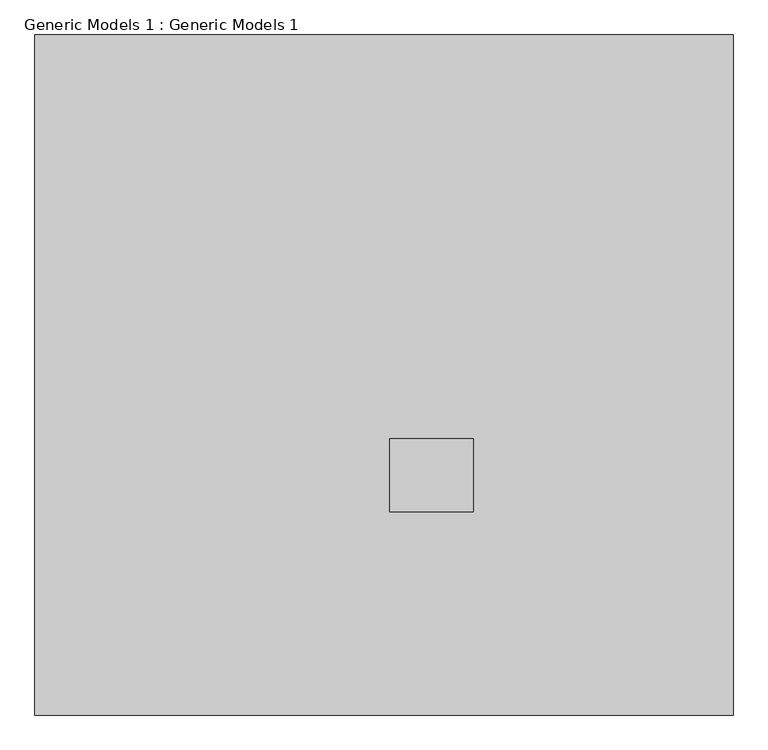
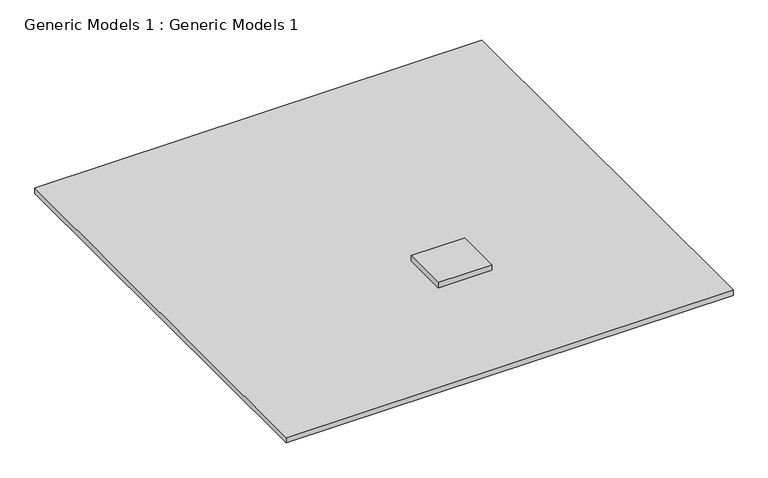
"""IFC4 building model written with IfcOpenShell, lengths in millimetres: proxy geometry, Generic Models 1 : Generic Models 1."""

from ifc_helpers import new_model, si_unit, frame, origin, origin_with_axes, place, context, project, spatial, polyline, outline, extrude, source, transform, mapped, element, save


def generic_models_1_generic_models_1_010c0d49(model_context):
    return source(origin(), model_context, "Body", "SweptSolid", [
        extrude(outline(polyline([(1074.6746771, 1256.1715228), (1074.6746771, -21706.0341115), (-22498.0233478, -21706.0341115), (-22498.0233478, 1256.1715228), (1074.6746771, 1256.1715228)])), frame((0.0, 0.0, -304.8), z_axis=(0.0, 0.0, 1.0), x_axis=(1.0, 0.0, 0.0)), (0.0, 0.0, 1.0), 304.8),
        extrude(outline(polyline([(-7700.6281629, -12372.4678064), (-7700.6281629, -14848.9678064), (-10520.0281629, -14848.9678064), (-10520.0281629, -12372.4678064), (-7700.6281629, -12372.4678064)])), origin_with_axes(), (0.0, 0.0, 1.0), 304.8),
    ])


if __name__ == "__main__":
    model = new_model("IFC4")
    model_context = context("Model", 3, world=origin())
    ifc_project = project(units=[si_unit("LENGTHUNIT", "METRE", prefix="MILLI")], contexts=[model_context])
    site = spatial("IfcSite", under=ifc_project)
    building = spatial("IfcBuilding", under=site)
    placement = place(None, origin())
    generic_models_1_generic_models_1_shape = generic_models_1_generic_models_1_010c0d49(model_context)
    element("IfcBuildingElementProxy", 1, Name="Generic Models 1 : Generic Models 1", ObjectType="Generic Models 1 : Generic Models 1", at=placement, inside=building, context=model_context, shape_type="MappedRepresentation", body=[
        mapped(generic_models_1_generic_models_1_shape, transform((0.0, 0.0, 0.0), x_axis=(1.0, 0.0, 0.0), y_axis=(0.0, 1.0, 0.0), z_axis=(0.0, 0.0, 1.0))),
    ])
    save(model, "model.ifc")
